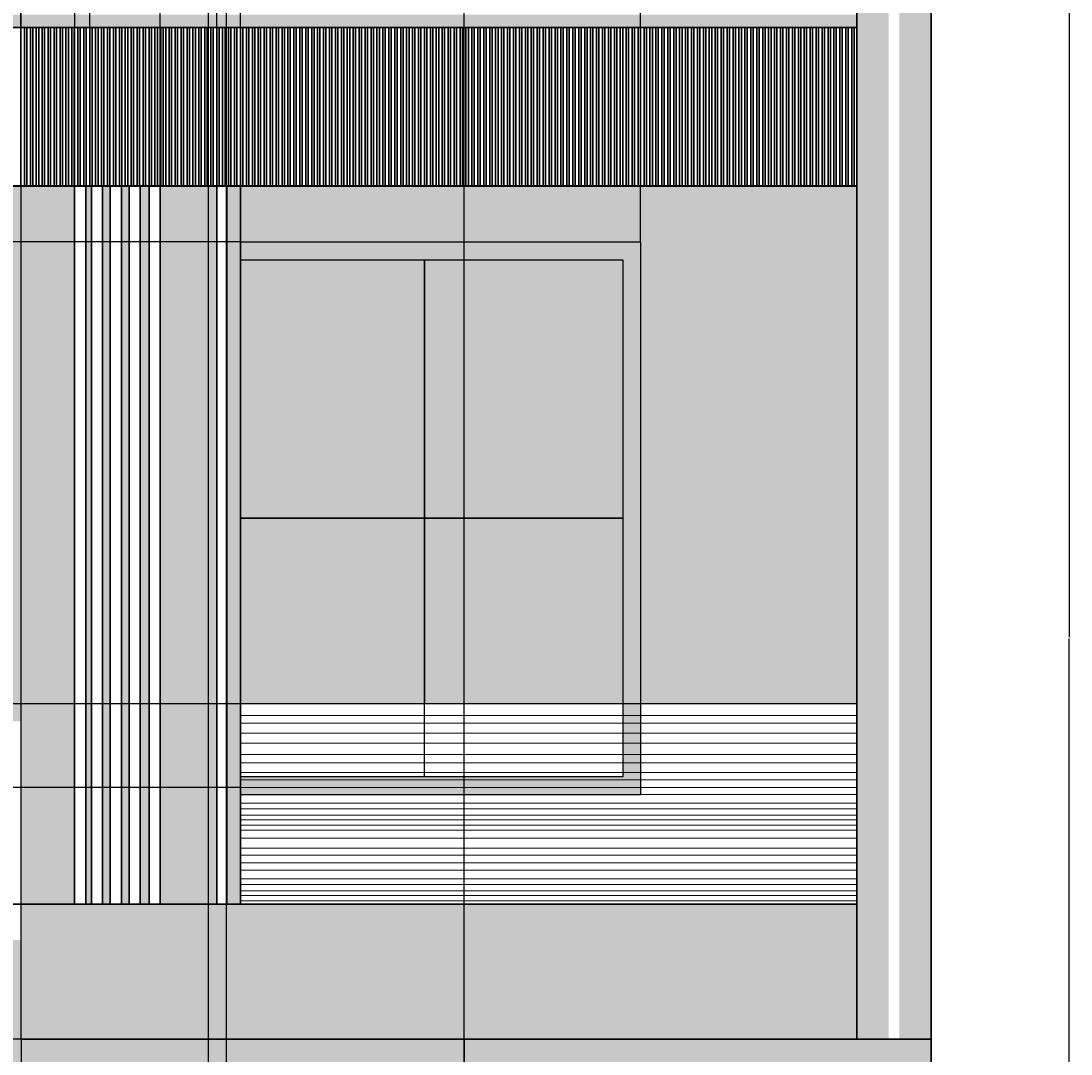
# Model space of a CAD drawing. Units: feet. Extents: x 2368 to 2738, y 1285 to 1782.
# Tile 5 of 6: x 2561 to 2738, y 1464 to 1638. Entities that reach past the tile are written whole.
import ezdxf

# ---------------------------------------------------------------- set-up
doc = ezdxf.new("R2010")
doc.units = ezdxf.units.FT
for name, color, linetype, lineweight in [('A-ANNO-DIMS', 2, 'Continuous', 18), ('A-ELEV', 7, 'Continuous', 35), ('A-ELEV-PATT', 252, 'Continuous', 13), ('A-FLOR-HRAL', 8, 'Continuous', 18), ('A-GLAZ', 4, 'Continuous', 25)]:
    doc.layers.add(name, color=color, linetype=linetype, lineweight=lineweight)
doc.styles.get("Standard").update_dxf_attribs({"font": 'arial.ttf'})
doc.dimstyles.get("Standard").update_dxf_attribs({"dimtxt": 0.18, "dimasz": 0.18, "dimexe": 0.18, "dimexo": 0.0625, "dimgap": 0.09, "dimtad": 0, "dimtih": 1, "dimtoh": 1, "dimdec": 1, "dimzin": 0, "dimdsep": 46, "dimlunit": 3, "dimtxsty": 'Standard', "dimcen": 0.09, "dimadec": 0, "dimazin": 0, "dimtfac": 1, "dimtdec": 1, "dimtofl": 0, "dimtmove": 0, "dimatfit": 3, "dimfxl": 1, "dimtolj": 1, "dimtzin": 0, "dimarcsym": 0})

# ---------------------------------------------------------------- blocks, each defined once
blk = doc.blocks.new('*D2')
at = {"layer": 'A-ANNO-DIMS', "color": 0, "lineweight": -2, "transparency": 16777216}
for p, q in [((2714.23, 1758.68), (2737.59, 1758.68)), ((2737.41, 1758.5), (2737.41, 1533.95)), ((2737.41, 1309.04), (2737.41, 1533.58)), ((2714.23, 1308.86), (2737.59, 1308.86))]:
    blk.add_line(p, q, dxfattribs=at)
at = {"layer": 'A-ANNO-DIMS', "color": 0, "transparency": 16777216}
for points in [[(2737.38, 1758.5), (2737.44, 1758.5), (2737.41, 1758.68)], [(2737.38, 1309.04), (2737.44, 1309.04), (2737.41, 1308.86)]]:
    blk.add_solid(points, dxfattribs=at)
at = {"layer": 'Defpoints', "color": 0, "transparency": 16777216}
for p in [(2714.16, 1758.68), (2737.41, 1758.68), (2714.16, 1308.86)]:
    blk.add_point(p, dxfattribs=at)
at = {"layer": 'A-ANNO-DIMS', "color": 0, "transparency": 16777216, "insert": (2737.41, 1533.77), "char_height": 0.18, "attachment_point": 5}
blk.add_mtext('\\A1;449.8', dxfattribs=at)
blk = doc.blocks.new('*D19')
at = {"layer": 'A-ANNO-DIMS', "color": 0, "lineweight": -2, "transparency": 16777216}
for p, q in [((2560.8, 1466.04), (2560.8, 1285.43)), ((2543.45, 1350.79), (2543.45, 1285.43)), ((2543.63, 1285.61), (2551.74, 1285.61)), ((2560.62, 1285.61), (2552.51, 1285.61))]:
    blk.add_line(p, q, dxfattribs=at)
at = {"layer": 'A-ANNO-DIMS', "color": 0, "transparency": 16777216}
for points in [[(2543.63, 1285.64), (2543.63, 1285.58), (2543.45, 1285.61)], [(2560.62, 1285.64), (2560.62, 1285.58), (2560.8, 1285.61)]]:
    blk.add_solid(points, dxfattribs=at)
at = {"layer": 'Defpoints', "color": 0, "transparency": 16777216}
for p in [(2560.8, 1466.1), (2543.45, 1350.86), (2560.8, 1285.61)]:
    blk.add_point(p, dxfattribs=at)
at = {"layer": 'A-ANNO-DIMS', "color": 0, "transparency": 16777216, "insert": (2552.12, 1285.61), "char_height": 0.18, "attachment_point": 5}
blk.add_mtext('\\A1;17.35', dxfattribs=at)
blk = doc.blocks.new('*D20')
at = {"layer": 'A-ANNO-DIMS', "color": 0, "lineweight": -2, "transparency": 16777216}
for p, q in [((2560.8, 1466.04), (2560.8, 1285.43)), ((2592.41, 1367.92), (2592.41, 1285.43)), ((2560.98, 1285.61), (2576.21, 1285.61)), ((2592.23, 1285.61), (2577, 1285.61))]:
    blk.add_line(p, q, dxfattribs=at)
at = {"layer": 'A-ANNO-DIMS', "color": 0, "transparency": 16777216}
for points in [[(2560.98, 1285.64), (2560.98, 1285.58), (2560.8, 1285.61)], [(2592.23, 1285.64), (2592.23, 1285.58), (2592.41, 1285.61)]]:
    blk.add_solid(points, dxfattribs=at)
at = {"layer": 'Defpoints', "color": 0, "transparency": 16777216}
for p in [(2560.8, 1466.1), (2592.41, 1367.98), (2592.41, 1285.61)]:
    blk.add_point(p, dxfattribs=at)
at = {"layer": 'A-ANNO-DIMS', "color": 0, "transparency": 16777216, "insert": (2576.6, 1285.61), "char_height": 0.18, "attachment_point": 5}
blk.add_mtext('\\A1;31.62', dxfattribs=at)
blk = doc.blocks.new('*D33')
at = {"layer": 'A-ANNO-DIMS', "color": 0, "lineweight": -2, "transparency": 16777216}
for p, q in [((2592.41, 1461.2), (2592.41, 1782.11)), ((2592.59, 1781.93), (2593.76, 1781.93)), ((2595.23, 1781.93), (2594.06, 1781.93)), ((2595.41, 1458.2), (2595.41, 1782.11))]:
    blk.add_line(p, q, dxfattribs=at)
at = {"layer": 'A-ANNO-DIMS', "color": 0, "transparency": 16777216}
for points in [[(2592.59, 1781.96), (2592.59, 1781.9), (2592.41, 1781.93)], [(2595.23, 1781.96), (2595.23, 1781.9), (2595.41, 1781.93)]]:
    blk.add_solid(points, dxfattribs=at)
at = {"layer": 'Defpoints', "color": 0, "transparency": 16777216}
for p in [(2595.41, 1781.93), (2592.41, 1461.14), (2595.41, 1458.14)]:
    blk.add_point(p, dxfattribs=at)
at = {"layer": 'A-ANNO-DIMS', "color": 0, "transparency": 16777216, "insert": (2593.91, 1781.93), "char_height": 0.18, "attachment_point": 5}
blk.add_mtext('\\A1;3', dxfattribs=at)
blk = doc.blocks.new('*D34')
at = {"layer": 'A-ANNO-DIMS', "color": 0, "lineweight": -2, "transparency": 16777216}
for p, q in [((2560.8, 1466.16), (2560.8, 1782.11)), ((2560.98, 1781.93), (2597.75, 1781.93)), ((2635.31, 1781.93), (2598.54, 1781.93)), ((2635.49, 1466.16), (2635.49, 1782.11))]:
    blk.add_line(p, q, dxfattribs=at)
at = {"layer": 'A-ANNO-DIMS', "color": 0, "transparency": 16777216}
for points in [[(2560.98, 1781.96), (2560.98, 1781.9), (2560.8, 1781.93)], [(2635.31, 1781.96), (2635.31, 1781.9), (2635.49, 1781.93)]]:
    blk.add_solid(points, dxfattribs=at)
at = {"layer": 'Defpoints', "color": 0, "transparency": 16777216}
for p in [(2635.49, 1781.93), (2560.8, 1466.1), (2635.49, 1466.1)]:
    blk.add_point(p, dxfattribs=at)
at = {"layer": 'A-ANNO-DIMS', "color": 0, "transparency": 16777216, "insert": (2598.14, 1781.93), "char_height": 0.18, "attachment_point": 5}
blk.add_mtext('\\A1;74.69', dxfattribs=at)
blk = doc.blocks.new('*D35')
at = {"layer": 'A-ANNO-DIMS', "color": 0, "lineweight": -2, "transparency": 16777216}
for p, q in [((2635.49, 1466.16), (2635.49, 1782.11)), ((2635.67, 1781.93), (2668.18, 1781.93)), ((2701.48, 1781.93), (2668.97, 1781.93)), ((2701.66, 1466.16), (2701.66, 1782.11))]:
    blk.add_line(p, q, dxfattribs=at)
at = {"layer": 'A-ANNO-DIMS', "color": 0, "transparency": 16777216}
for points in [[(2635.67, 1781.96), (2635.67, 1781.9), (2635.49, 1781.93)], [(2701.48, 1781.96), (2701.48, 1781.9), (2701.66, 1781.93)]]:
    blk.add_solid(points, dxfattribs=at)
at = {"layer": 'Defpoints', "color": 0, "transparency": 16777216}
for p in [(2701.66, 1781.93), (2635.49, 1466.1), (2701.66, 1466.1)]:
    blk.add_point(p, dxfattribs=at)
at = {"layer": 'A-ANNO-DIMS', "color": 0, "transparency": 16777216, "insert": (2668.57, 1781.93), "char_height": 0.18, "attachment_point": 5}
blk.add_mtext('\\A1;66.17', dxfattribs=at)
blk = doc.blocks.new('*D36')
at = {"layer": 'A-ANNO-DIMS', "color": 0, "lineweight": -2, "transparency": 16777216}
for p, q in [((2701.6, 1488.86), (2368.11, 1488.86)), ((2368.29, 1488.68), (2368.29, 1477.66)), ((2368.29, 1466.28), (2368.29, 1477.3)), ((2701.6, 1466.1), (2368.11, 1466.1))]:
    blk.add_line(p, q, dxfattribs=at)
at = {"layer": 'A-ANNO-DIMS', "color": 0, "transparency": 16777216}
for points in [[(2368.26, 1488.68), (2368.32, 1488.68), (2368.29, 1488.86)], [(2368.26, 1466.28), (2368.32, 1466.28), (2368.29, 1466.1)]]:
    blk.add_solid(points, dxfattribs=at)
at = {"layer": 'Defpoints', "color": 0, "transparency": 16777216}
for p in [(2368.29, 1488.86), (2701.66, 1488.86), (2701.66, 1466.1)]:
    blk.add_point(p, dxfattribs=at)
at = {"layer": 'A-ANNO-DIMS', "color": 0, "transparency": 16777216, "insert": (2368.29, 1477.48), "char_height": 0.18, "attachment_point": 5}
blk.add_mtext('\\A1;22.754', dxfattribs=at)
blk = doc.blocks.new('*D37')
at = {"layer": 'A-ANNO-DIMS', "color": 0, "lineweight": -2, "transparency": 16777216}
for p, q in [((2701.6, 1522.63), (2368.11, 1522.63)), ((2368.29, 1522.45), (2368.29, 1505.93)), ((2368.29, 1489.04), (2368.29, 1505.56)), ((2701.6, 1488.86), (2368.11, 1488.86))]:
    blk.add_line(p, q, dxfattribs=at)
at = {"layer": 'A-ANNO-DIMS', "color": 0, "transparency": 16777216}
for points in [[(2368.26, 1522.45), (2368.32, 1522.45), (2368.29, 1522.63)], [(2368.26, 1489.04), (2368.32, 1489.04), (2368.29, 1488.86)]]:
    blk.add_solid(points, dxfattribs=at)
at = {"layer": 'Defpoints', "color": 0, "transparency": 16777216}
for p in [(2368.29, 1522.63), (2701.66, 1522.63), (2701.66, 1488.86)]:
    blk.add_point(p, dxfattribs=at)
at = {"layer": 'A-ANNO-DIMS', "color": 0, "transparency": 16777216, "insert": (2368.29, 1505.74), "char_height": 0.18, "attachment_point": 5}
blk.add_mtext('\\A1;33.776', dxfattribs=at)
blk = doc.blocks.new('*D38')
at = {"layer": 'A-ANNO-DIMS', "color": 0, "lineweight": -2, "transparency": 16777216}
for p, q in [((2701.6, 1636.62), (2368.11, 1636.62)), ((2368.29, 1636.44), (2368.29, 1623.45)), ((2368.29, 1610.09), (2368.29, 1623.08)), ((2701.6, 1609.91), (2368.11, 1609.91))]:
    blk.add_line(p, q, dxfattribs=at)
at = {"layer": 'A-ANNO-DIMS', "color": 0, "transparency": 16777216}
for points in [[(2368.26, 1636.44), (2368.32, 1636.44), (2368.29, 1636.62)], [(2368.26, 1610.09), (2368.32, 1610.09), (2368.29, 1609.91)]]:
    blk.add_solid(points, dxfattribs=at)
at = {"layer": 'Defpoints', "color": 0, "transparency": 16777216}
for p in [(2368.29, 1636.62), (2701.66, 1636.62), (2701.66, 1609.91)]:
    blk.add_point(p, dxfattribs=at)
at = {"layer": 'A-ANNO-DIMS', "color": 0, "transparency": 16777216, "insert": (2368.29, 1623.26), "char_height": 0.18, "attachment_point": 5}
blk.add_mtext('\\A1;26.72', dxfattribs=at)
blk = doc.blocks.new('*D54')
at = {"layer": 'A-ANNO-DIMS', "color": 0, "lineweight": -2, "transparency": 16777216}
for p, q in [((2560.78, 1609.97), (2560.78, 1782.11)), ((2560.96, 1781.93), (2564.98, 1781.93)), ((2569.66, 1781.93), (2565.63, 1781.93)), ((2569.84, 1609.97), (2569.84, 1782.11))]:
    blk.add_line(p, q, dxfattribs=at)
at = {"layer": 'A-ANNO-DIMS', "color": 0, "transparency": 16777216}
for points in [[(2560.96, 1781.96), (2560.96, 1781.9), (2560.78, 1781.93)], [(2569.66, 1781.96), (2569.66, 1781.9), (2569.84, 1781.93)]]:
    blk.add_solid(points, dxfattribs=at)
at = {"layer": 'Defpoints', "color": 0, "transparency": 16777216}
for p in [(2569.84, 1781.93), (2560.78, 1609.91), (2569.84, 1609.91)]:
    blk.add_point(p, dxfattribs=at)
at = {"layer": 'A-ANNO-DIMS', "color": 0, "transparency": 16777216, "insert": (2565.31, 1781.93), "char_height": 0.18, "attachment_point": 5}
blk.add_mtext('\\A1;9.06', dxfattribs=at)
blk = doc.blocks.new('*D55')
at = {"layer": 'A-ANNO-DIMS', "color": 0, "lineweight": -2, "transparency": 16777216}
for p, q in [((2569.84, 1609.97), (2569.84, 1782.11)), ((2570.02, 1781.93), (2576.72, 1781.93)), ((2584.06, 1781.93), (2577.35, 1781.93)), ((2584.24, 1609.97), (2584.24, 1782.11))]:
    blk.add_line(p, q, dxfattribs=at)
at = {"layer": 'A-ANNO-DIMS', "color": 0, "transparency": 16777216}
for points in [[(2570.02, 1781.96), (2570.02, 1781.9), (2569.84, 1781.93)], [(2584.06, 1781.96), (2584.06, 1781.9), (2584.24, 1781.93)]]:
    blk.add_solid(points, dxfattribs=at)
at = {"layer": 'Defpoints', "color": 0, "transparency": 16777216}
for p in [(2584.24, 1781.93), (2569.84, 1609.91), (2584.24, 1609.91)]:
    blk.add_point(p, dxfattribs=at)
at = {"layer": 'A-ANNO-DIMS', "color": 0, "transparency": 16777216, "insert": (2577.04, 1781.93), "char_height": 0.18, "attachment_point": 5}
blk.add_mtext('\\A1;14.4', dxfattribs=at)
blk = doc.blocks.new('*D56')
at = {"layer": 'A-ANNO-DIMS', "color": 0, "lineweight": -2, "transparency": 16777216}
for p, q in [((2593.78, 1609.97), (2593.78, 1782.11)), ((2593.96, 1781.93), (2595.62, 1781.93)), ((2597.6, 1781.93), (2595.93, 1781.93)), ((2597.78, 1609.97), (2597.78, 1782.11))]:
    blk.add_line(p, q, dxfattribs=at)
at = {"layer": 'A-ANNO-DIMS', "color": 0, "transparency": 16777216}
for points in [[(2593.96, 1781.96), (2593.96, 1781.9), (2593.78, 1781.93)], [(2597.6, 1781.96), (2597.6, 1781.9), (2597.78, 1781.93)]]:
    blk.add_solid(points, dxfattribs=at)
at = {"layer": 'Defpoints', "color": 0, "transparency": 16777216}
for p in [(2597.78, 1781.93), (2593.78, 1609.91), (2597.78, 1609.91)]:
    blk.add_point(p, dxfattribs=at)
at = {"layer": 'A-ANNO-DIMS', "color": 0, "transparency": 16777216, "insert": (2595.78, 1781.93), "char_height": 0.18, "attachment_point": 5}
blk.add_mtext('\\A1;4', dxfattribs=at)
blk = doc.blocks.new('*D57')
at = {"layer": 'A-ANNO-DIMS', "color": 0, "lineweight": -2, "transparency": 16777216}
for p, q in [((2569.84, 1609.97), (2569.84, 1782.11)), ((2570.02, 1781.93), (2570.71, 1781.93)), ((2572.19, 1781.93), (2571.5, 1781.93)), ((2572.37, 1609.97), (2572.37, 1782.11))]:
    blk.add_line(p, q, dxfattribs=at)
at = {"layer": 'A-ANNO-DIMS', "color": 0, "transparency": 16777216}
for points in [[(2570.02, 1781.96), (2570.02, 1781.9), (2569.84, 1781.93)], [(2572.19, 1781.96), (2572.19, 1781.9), (2572.37, 1781.93)]]:
    blk.add_solid(points, dxfattribs=at)
at = {"layer": 'Defpoints', "color": 0, "transparency": 16777216}
for p in [(2572.37, 1781.93), (2569.84, 1609.91), (2572.37, 1609.91)]:
    blk.add_point(p, dxfattribs=at)
at = {"layer": 'A-ANNO-DIMS', "color": 0, "transparency": 16777216, "insert": (2571.11, 1781.93), "char_height": 0.18, "attachment_point": 5}
blk.add_mtext('\\A1;2.539', dxfattribs=at)
blk = doc.blocks.new('*D58')
at = {"layer": 'A-ANNO-DIMS', "color": 0, "lineweight": -2, "transparency": 16777216}
for p, q in [((2597.78, 1600.54), (2597.78, 1782.11)), ((2597.96, 1781.93), (2631.09, 1781.93)), ((2665.02, 1781.93), (2631.88, 1781.93)), ((2665.2, 1600.54), (2665.2, 1782.11))]:
    blk.add_line(p, q, dxfattribs=at)
at = {"layer": 'A-ANNO-DIMS', "color": 0, "transparency": 16777216}
for points in [[(2597.96, 1781.96), (2597.96, 1781.9), (2597.78, 1781.93)], [(2665.02, 1781.96), (2665.02, 1781.9), (2665.2, 1781.93)]]:
    blk.add_solid(points, dxfattribs=at)
at = {"layer": 'Defpoints', "color": 0, "transparency": 16777216}
for p in [(2665.2, 1781.93), (2597.78, 1600.48), (2665.2, 1600.48)]:
    blk.add_point(p, dxfattribs=at)
at = {"layer": 'A-ANNO-DIMS', "color": 0, "transparency": 16777216, "insert": (2631.49, 1781.93), "char_height": 0.18, "attachment_point": 5}
blk.add_mtext('\\A1;67.42', dxfattribs=at)
blk = doc.blocks.new('*D59')
at = {"layer": 'A-ANNO-DIMS', "color": 0, "lineweight": -2, "transparency": 16777216}
for p, q in [((2665.2, 1600.54), (2665.2, 1782.11)), ((2665.38, 1781.93), (2683.03, 1781.93)), ((2701.48, 1781.93), (2683.82, 1781.93)), ((2701.66, 1609.97), (2701.66, 1782.11))]:
    blk.add_line(p, q, dxfattribs=at)
at = {"layer": 'A-ANNO-DIMS', "color": 0, "transparency": 16777216}
for points in [[(2665.38, 1781.96), (2665.38, 1781.9), (2665.2, 1781.93)], [(2701.48, 1781.96), (2701.48, 1781.9), (2701.66, 1781.93)]]:
    blk.add_solid(points, dxfattribs=at)
at = {"layer": 'Defpoints', "color": 0, "transparency": 16777216}
for p in [(2701.66, 1781.93), (2701.66, 1609.91), (2665.2, 1600.48)]:
    blk.add_point(p, dxfattribs=at)
at = {"layer": 'A-ANNO-DIMS', "color": 0, "transparency": 16777216, "insert": (2683.43, 1781.93), "char_height": 0.18, "attachment_point": 5}
blk.add_mtext('\\A1;36.46', dxfattribs=at)
blk = doc.blocks.new('*D60')
at = {"layer": 'A-ANNO-DIMS', "color": 0, "lineweight": -2, "transparency": 16777216}
for p, q in [((2597.71, 1600.48), (2368.11, 1600.48)), ((2368.29, 1600.3), (2368.29, 1554.7)), ((2368.29, 1508.74), (2368.29, 1554.34)), ((2597.71, 1508.56), (2368.11, 1508.56))]:
    blk.add_line(p, q, dxfattribs=at)
at = {"layer": 'A-ANNO-DIMS', "color": 0, "transparency": 16777216}
for points in [[(2368.26, 1600.3), (2368.32, 1600.3), (2368.29, 1600.48)], [(2368.26, 1508.74), (2368.32, 1508.74), (2368.29, 1508.56)]]:
    blk.add_solid(points, dxfattribs=at)
at = {"layer": 'Defpoints', "color": 0, "transparency": 16777216}
for p in [(2368.29, 1600.48), (2597.78, 1600.48), (2597.78, 1508.56)]:
    blk.add_point(p, dxfattribs=at)
at = {"layer": 'A-ANNO-DIMS', "color": 0, "transparency": 16777216, "insert": (2368.29, 1554.52), "char_height": 0.18, "attachment_point": 5}
blk.add_mtext('\\A1;91.92', dxfattribs=at)

msp = doc.modelspace()

# ---------------------------------------------------------------- hatches: boundary and pattern name
at = {"layer": 'A-ELEV-PATT'}
h = msp.add_hatch(color=256, dxfattribs=at)
h.set_gradient(color1=(192, 192, 192), color2=(192, 192, 192), tint=1)
h.paths.add_polyline_path([(2714.1625, 1758.6751), (2519.621, 1758.6751), (2519.621, 1716.8552), (2714.1625, 1716.8552)])
h.paths.add_polyline_path([(2701.6591, 1693.9847), (2714.1625, 1693.9847), (2714.1625, 1710.8552), (2519.621, 1710.8552), (2519.621, 1662.8552), (2592.4132, 1662.8552), (2592.4132, 1689.493), (2665.1962, 1689.493), (2665.1962, 1662.8552), (2701.6591, 1662.8552)])
h.paths.add_polyline_path([(2701.6591, 1609.9058), (2597.776, 1609.9058), (2597.776, 1600.4784), (2665.1962, 1600.4784), (2665.1962, 1596.3371), (2665.1962, 1522.6314), (2701.6591, 1522.6314)])
h.paths.add_polyline_path([(2463.0324, 1598.097), (2536.677, 1598.097), (2536.677, 1519.7115), (2560.74, 1519.7115), (2560.5754, 1609.9058), (2542.3749, 1609.9058), (2441.2488, 1609.9058), (2441.2488, 1519.7115), (2463.0324, 1519.7115)])
h.paths.add_polyline_path([(2506.1956, 1662.8552), (2391.5414, 1662.8552), (2391.5414, 1644.4206), (2438.815, 1644.4206, -0.34592239), (2445.9507, 1638.8128), (2506.1956, 1638.8128)])
h.paths.add_polyline_path([(2410.9473, 1609.9058, -0.04175491), (2411.9608, 1614.8552), (2391.5414, 1614.8552), (2391.5414, 1488.8552), (2410.9473, 1488.8552)])
h.paths.add_polyline_path([(2426.5897, 1605.0962, 1), (2422.7862, 1605.0962), (2422.7862, 1509.5049, 1), (2426.5897, 1509.5049)])
h.paths.add_polyline_path([(2463.0324, 1460.097), (2536.677, 1460.097), (2536.677, 1350.8552), (2543.4468, 1350.8552), (2543.4468, 1482.8552), (2391.5414, 1482.8552), (2391.5414, 1350.8552), (2463.0324, 1350.8552)])
h.paths.add_polyline_path([(2436.8485, 1456.084), (2436.8485, 1379.669), (2399.9065, 1379.669), (2399.9065, 1456.084)], flags=16)
h.paths.add_polyline_path([(2434.8485, 1454.084), (2434.8485, 1381.669), (2401.9065, 1381.669), (2401.9065, 1454.084)], flags=0)
h.paths.add_polyline_path([(2714.1625, 1350.8552), (2391.5414, 1350.8552), (2391.5414, 1320.8552), (2714.1625, 1320.8552)])
h.paths.add_polyline_path([(2714.1625, 1320.8552), (2391.5414, 1320.8552), (2391.5414, 1308.8552), (2714.1625, 1308.8552)])
h = msp.add_hatch(color=256, dxfattribs=at)
h.set_gradient(color1=(128, 128, 128), color2=(128, 128, 128), tint=1)
h.paths.add_polyline_path([(2519.621, 1716.8552), (2409.5414, 1716.8552), (2409.5414, 1662.8552), (2415.5414, 1662.8552), (2415.5414, 1710.8552), (2519.621, 1710.8552)])
h.paths.add_polyline_path([(2714.1625, 1716.8552), (2519.621, 1716.8552), (2519.621, 1710.8552), (2714.1625, 1710.8552)])
h.paths.add_polyline_path([(2701.6591, 1638.8128), (2445.9507, 1638.8128, -0.0752442), (2446.1448, 1636.6235), (2542.3749, 1636.6235), (2542.776, 1636.6235), (2701.6591, 1636.6235)])
h = msp.add_hatch(color=256, dxfattribs=at)
h.set_gradient(color1=(255, 255, 255), tint=1)
h.paths.add_polyline_path([(2714.1625, 1693.9847), (2708.7975, 1693.9847), (2708.7975, 1466.101), (2714.1625, 1466.101)])
h.paths.add_polyline_path([(2707.0241, 1693.9847), (2701.6591, 1693.9847), (2701.6591, 1466.101), (2707.0241, 1466.101)])
h = msp.add_hatch(color=256, dxfattribs=at)
h.set_gradient(color1=(255, 255, 255), tint=1)
h.paths.add_polyline_path([(2595.4132, 1686.493), (2662.1962, 1686.493), (2662.1962, 1662.8552), (2665.1962, 1662.8552), (2665.1962, 1689.493), (2592.4132, 1689.493), (2592.4132, 1662.8552), (2595.4132, 1662.8552)])
h.paths.add_polyline_path([(2665.1962, 1600.4784), (2597.776, 1600.4784), (2597.776, 1597.4784), (2662.1962, 1597.4784), (2662.1962, 1510.3225), (2597.776, 1510.3225), (2597.776, 1507.3225), (2665.1962, 1507.3225)])
h.paths.add_polyline_path([(2665.1962, 1461.1396), (2592.4132, 1461.1396), (2592.4132, 1367.9838), (2665.1962, 1367.9838)])
h.paths.add_polyline_path([(2662.1962, 1458.1396), (2662.1962, 1370.9838), (2595.4132, 1370.9838), (2595.4132, 1458.1396)], flags=16)
h.paths.add_polyline_path([(2593.776, 1609.9058), (2584.2358, 1609.9058), (2584.2358, 1488.8552), (2593.776, 1488.8552)])
h.paths.add_polyline_path([(2597.776, 1609.9058), (2595.4517, 1609.9058), (2595.4517, 1488.8552), (2597.776, 1488.8552)])
h.paths.add_polyline_path([(2569.8357, 1609.9058), (2560.5754, 1609.9058), (2560.74, 1519.7115), (2560.7407, 1519.7115), (2560.7407, 1519.3328), (2560.7963, 1488.8552), (2569.8357, 1488.8552)])
h.paths.add_polyline_path([(2572.6807, 1609.9058), (2571.6967, 1609.9058), (2571.6967, 1488.8552), (2572.6807, 1488.8552)])
h.paths.add_polyline_path([(2575.8428, 1609.9058), (2574.5416, 1609.9058), (2574.5416, 1488.8552), (2575.8428, 1488.8552)])
h.paths.add_polyline_path([(2579.0308, 1609.9058), (2577.7037, 1609.9058), (2577.7037, 1488.8552), (2579.0308, 1488.8552)])
h.paths.add_polyline_path([(2582.3749, 1609.9058), (2580.8918, 1609.9058), (2580.8918, 1488.8552), (2582.3749, 1488.8552)])
h = msp.add_hatch(color=256, dxfattribs=at)
h.set_gradient(color1=(0, 255, 255), color2=(0, 255, 255), tint=1)
h.paths.add_polyline_path([(2418.2281, 1454.084), (2401.9065, 1454.084), (2401.9065, 1381.669), (2418.2281, 1381.669)])
h.paths.add_polyline_path([(2434.8485, 1454.084), (2418.5148, 1454.084), (2418.5148, 1381.669), (2434.8485, 1381.669)])
h.paths.add_polyline_path([(2662.1962, 1458.1396), (2595.4132, 1458.1396), (2595.4132, 1414.5617), (2662.1962, 1414.5617)])
h.paths.add_polyline_path([(2662.1962, 1414.5617), (2628.8047, 1414.5617), (2628.8047, 1370.9838), (2662.1962, 1370.9838)])
h.paths.add_polyline_path([(2628.8047, 1414.5617), (2595.4132, 1414.5617), (2595.4132, 1370.9838), (2628.8047, 1370.9838)])
h.paths.add_polyline_path([(2662.1962, 1597.4784), (2628.8047, 1597.4784), (2628.8047, 1553.9004), (2662.1962, 1553.9004)])
h.paths.add_polyline_path([(2628.8047, 1597.4784), (2597.776, 1597.4784), (2597.776, 1553.9004), (2628.8047, 1553.9004)])
h.paths.add_polyline_path([(2628.8047, 1553.9004), (2597.776, 1553.9004), (2597.776, 1522.6314), (2628.8047, 1522.6314)])
h.paths.add_polyline_path([(2662.1962, 1553.9004), (2628.8047, 1553.9004), (2628.8047, 1522.6314), (2662.1962, 1522.6314)])
h.paths.add_polyline_path([(2662.1962, 1686.493), (2628.8047, 1686.493), (2628.8047, 1662.8552), (2662.1962, 1662.8552)])
h.paths.add_polyline_path([(2628.8047, 1686.493), (2595.4132, 1686.493), (2595.4132, 1662.8552), (2628.8047, 1662.8552)])
h = msp.add_hatch(color=256, dxfattribs=at)
h.set_gradient(color1=(242, 242, 242), color2=(242, 242, 242), tint=1)
h.paths.add_polyline_path([(2542.3749, 1636.6235), (2440.8236, 1636.6235, 0.37790365), (2410.9473, 1609.9058), (2410.9473, 1488.8552), (2441.2488, 1488.8552), (2441.2488, 1609.9058), (2542.3749, 1609.9058)])
h.paths.add_polyline_path([(2426.5897, 1605.0962), (2426.5897, 1509.5049, -1), (2422.7862, 1509.5049), (2422.7862, 1605.0962, -1)], flags=16)
h.paths.add_polyline_path([(2441.2488, 1636.6235), (2446.1448, 1636.6235, 0.43242195), (2438.815, 1644.4206), (2391.5414, 1644.4206), (2391.5414, 1620.8552), (2391.5414, 1614.8552), (2411.9608, 1614.8552, -0.33482359)])
h.paths.add_polyline_path([(2592.4132, 1461.1396), (2635.4878, 1461.1396), (2635.4878, 1466.101), (2560.7963, 1466.101), (2560.7963, 1482.8552), (2543.4468, 1482.8552), (2543.4468, 1350.8552), (2635.4878, 1350.8552), (2635.4878, 1367.9838), (2592.4132, 1367.9838)])
h = msp.add_hatch(color=256, dxfattribs=at)
h.set_gradient(color1=(128, 128, 128), color2=(128, 128, 128), tint=1)
h.paths.add_polyline_path([(2701.6591, 1488.8552), (2560.7963, 1488.8552), (2560.7963, 1466.101), (2701.6591, 1466.101)])
h = msp.add_hatch(color=256, dxfattribs=at)
h.set_gradient(color1=(144, 103, 100), color2=(144, 103, 100), tint=1)
h.paths.add_polyline_path([(2714.1625, 1466.101), (2701.6591, 1466.101), (2635.4878, 1466.101), (2635.4878, 1461.1396), (2665.1962, 1461.1396), (2665.1962, 1367.9838), (2635.4878, 1367.9838), (2635.4878, 1350.8552), (2714.1625, 1350.8552)])

# ---------------------------------------------------------------- linework, layer by layer
at = {"layer": 'A-ELEV'}
for p, q in [((2701.6591, 1693.9847), (2701.6591, 1466.101)), ((2714.1625, 1466.101), (2714.1625, 1693.9847)), ((2446.1448, 1636.6235), (2701.6591, 1636.6235)), ((2542.3749, 1636.6235), (2701.6591, 1636.6235)), ((2441.2488, 1609.9058), (2701.6591, 1609.9058)), ((2542.3749, 1609.9058), (2701.6591, 1609.9058)), ((2597.776, 1609.9058), (2597.776, 1488.8552)), ((2391.5414, 1488.8552), (2701.6591, 1488.8552)), ((2391.5414, 1488.8552), (2701.6591, 1488.8552)), ((2560.7963, 1488.8552), (2701.6591, 1488.8552)), ((2701.6591, 1466.101), (2560.7963, 1466.101)), ((2560.7963, 1466.101), (2701.6591, 1466.101)), ((2635.4878, 1461.1396), (2635.4878, 1466.101)), ((2635.4878, 1466.101), (2635.4878, 1461.1396)), ((2701.6591, 1466.101), (2714.1625, 1466.101))]:
    msp.add_line(p, q, dxfattribs=at)
msp.add_lwpolyline([(2714.1625, 1716.8552), (2714.1625, 1308.8552)], dxfattribs=at)
for points in [[(2714.1625, 1693.9847), (2701.6591, 1693.9847), (2701.6591, 1466.101), (2714.1625, 1466.101)], [(2561.3749, 1636.6235), (2561.776, 1636.6235), (2561.776, 1609.9058), (2561.3749, 1609.9058)], [(2562.3749, 1636.6235), (2562.776, 1636.6235), (2562.776, 1609.9058), (2562.3749, 1609.9058)], [(2563.3749, 1636.6235), (2563.776, 1636.6235), (2563.776, 1609.9058), (2563.3749, 1609.9058)], [(2564.3749, 1636.6235), (2564.776, 1636.6235), (2564.776, 1609.9058), (2564.3749, 1609.9058)], [(2565.3749, 1636.6235), (2565.776, 1636.6235), (2565.776, 1609.9058), (2565.3749, 1609.9058)], [(2566.3749, 1636.6235), (2566.776, 1636.6235), (2566.776, 1609.9058), (2566.3749, 1609.9058)], [(2567.3749, 1636.6235), (2567.776, 1636.6235), (2567.776, 1609.9058), (2567.3749, 1609.9058)], [(2568.3749, 1636.6235), (2568.776, 1636.6235), (2568.776, 1609.9058), (2568.3749, 1609.9058)], [(2569.3749, 1636.6235), (2569.776, 1636.6235), (2569.776, 1609.9058), (2569.3749, 1609.9058)], [(2570.3749, 1636.6235), (2570.776, 1636.6235), (2570.776, 1609.9058), (2570.3749, 1609.9058)], [(2571.3749, 1636.6235), (2571.776, 1636.6235), (2571.776, 1609.9058), (2571.3749, 1609.9058)], [(2572.3749, 1636.6235), (2572.776, 1636.6235), (2572.776, 1609.9058), (2572.3749, 1609.9058)], [(2573.3749, 1636.6235), (2573.776, 1636.6235), (2573.776, 1609.9058), (2573.3749, 1609.9058)], [(2574.3749, 1636.6235), (2574.776, 1636.6235), (2574.776, 1609.9058), (2574.3749, 1609.9058)], [(2575.3749, 1636.6235), (2575.776, 1636.6235), (2575.776, 1609.9058), (2575.3749, 1609.9058)], [(2576.3749, 1636.6235), (2576.776, 1636.6235), (2576.776, 1609.9058), (2576.3749, 1609.9058)], [(2577.3749, 1636.6235), (2577.776, 1636.6235), (2577.776, 1609.9058), (2577.3749, 1609.9058)], [(2578.3749, 1636.6235), (2578.776, 1636.6235), (2578.776, 1609.9058), (2578.3749, 1609.9058)], [(2579.3749, 1636.6235), (2579.776, 1636.6235), (2579.776, 1609.9058), (2579.3749, 1609.9058)], [(2580.3749, 1636.6235), (2580.776, 1636.6235), (2580.776, 1609.9058), (2580.3749, 1609.9058)], [(2581.3749, 1636.6235), (2581.776, 1636.6235), (2581.776, 1609.9058), (2581.3749, 1609.9058)], [(2582.3749, 1636.6235), (2582.776, 1636.6235), (2582.776, 1609.9058), (2582.3749, 1609.9058)], [(2583.3749, 1636.6235), (2583.776, 1636.6235), (2583.776, 1609.9058), (2583.3749, 1609.9058)], [(2584.3749, 1636.6235), (2584.776, 1636.6235), (2584.776, 1609.9058), (2584.3749, 1609.9058)], [(2584.776, 1636.6235), (2585.1771, 1636.6235), (2585.1771, 1609.9058), (2584.776, 1609.9058)], [(2585.776, 1636.6235), (2586.1771, 1636.6235), (2586.1771, 1609.9058), (2585.776, 1609.9058)], [(2586.776, 1636.6235), (2587.1771, 1636.6235), (2587.1771, 1609.9058), (2586.776, 1609.9058)], [(2587.776, 1636.6235), (2588.1771, 1636.6235), (2588.1771, 1609.9058), (2587.776, 1609.9058)], [(2588.776, 1636.6235), (2589.1771, 1636.6235), (2589.1771, 1609.9058), (2588.776, 1609.9058)], [(2589.776, 1636.6235), (2590.1771, 1636.6235), (2590.1771, 1609.9058), (2589.776, 1609.9058)], [(2590.776, 1636.6235), (2591.1771, 1636.6235), (2591.1771, 1609.9058), (2590.776, 1609.9058)], [(2591.776, 1636.6235), (2592.1771, 1636.6235), (2592.1771, 1609.9058), (2591.776, 1609.9058)], [(2592.776, 1636.6235), (2593.1771, 1636.6235), (2593.1771, 1609.9058), (2592.776, 1609.9058)], [(2593.776, 1636.6235), (2594.1771, 1636.6235), (2594.1771, 1609.9058), (2593.776, 1609.9058)], [(2594.776, 1636.6235), (2595.1771, 1636.6235), (2595.1771, 1609.9058), (2594.776, 1609.9058)], [(2595.776, 1636.6235), (2596.1771, 1636.6235), (2596.1771, 1609.9058), (2595.776, 1609.9058)], [(2596.776, 1636.6235), (2597.1771, 1636.6235), (2597.1771, 1609.9058), (2596.776, 1609.9058)], [(2597.776, 1636.6235), (2598.1771, 1636.6235), (2598.1771, 1609.9058), (2597.776, 1609.9058)], [(2598.776, 1636.6235), (2599.1771, 1636.6235), (2599.1771, 1609.9058), (2598.776, 1609.9058)], [(2599.776, 1636.6235), (2600.1771, 1636.6235), (2600.1771, 1609.9058), (2599.776, 1609.9058)], [(2600.776, 1636.6235), (2601.1771, 1636.6235), (2601.1771, 1609.9058), (2600.776, 1609.9058)], [(2601.776, 1636.6235), (2602.1771, 1636.6235), (2602.1771, 1609.9058), (2601.776, 1609.9058)], [(2602.776, 1636.6235), (2603.1771, 1636.6235), (2603.1771, 1609.9058), (2602.776, 1609.9058)], [(2603.776, 1636.6235), (2604.1771, 1636.6235), (2604.1771, 1609.9058), (2603.776, 1609.9058)], [(2604.776, 1636.6235), (2605.1771, 1636.6235), (2605.1771, 1609.9058), (2604.776, 1609.9058)], [(2605.776, 1636.6235), (2606.1771, 1636.6235), (2606.1771, 1609.9058), (2605.776, 1609.9058)], [(2606.776, 1636.6235), (2607.1771, 1636.6235), (2607.1771, 1609.9058), (2606.776, 1609.9058)], [(2607.776, 1636.6235), (2608.1771, 1636.6235), (2608.1771, 1609.9058), (2607.776, 1609.9058)], [(2608.776, 1636.6235), (2609.1771, 1636.6235), (2609.1771, 1609.9058), (2608.776, 1609.9058)], [(2609.776, 1636.6235), (2610.1771, 1636.6235), (2610.1771, 1609.9058), (2609.776, 1609.9058)], [(2610.776, 1636.6235), (2611.1771, 1636.6235), (2611.1771, 1609.9058), (2610.776, 1609.9058)], [(2611.776, 1636.6235), (2612.1771, 1636.6235), (2612.1771, 1609.9058), (2611.776, 1609.9058)], [(2612.776, 1636.6235), (2613.1771, 1636.6235), (2613.1771, 1609.9058), (2612.776, 1609.9058)], [(2613.776, 1636.6235), (2614.1771, 1636.6235), (2614.1771, 1609.9058), (2613.776, 1609.9058)], [(2614.776, 1636.6235), (2615.1771, 1636.6235), (2615.1771, 1609.9058), (2614.776, 1609.9058)], [(2615.776, 1636.6235), (2616.1771, 1636.6235), (2616.1771, 1609.9058), (2615.776, 1609.9058)], [(2616.776, 1636.6235), (2617.1771, 1636.6235), (2617.1771, 1609.9058), (2616.776, 1609.9058)], [(2617.776, 1636.6235), (2618.1771, 1636.6235), (2618.1771, 1609.9058), (2617.776, 1609.9058)], [(2618.776, 1636.6235), (2619.1771, 1636.6235), (2619.1771, 1609.9058), (2618.776, 1609.9058)], [(2619.776, 1636.6235), (2620.1771, 1636.6235), (2620.1771, 1609.9058), (2619.776, 1609.9058)], [(2620.776, 1636.6235), (2621.1771, 1636.6235), (2621.1771, 1609.9058), (2620.776, 1609.9058)], [(2621.776, 1636.6235), (2622.1771, 1636.6235), (2622.1771, 1609.9058), (2621.776, 1609.9058)], [(2622.776, 1636.6235), (2623.1771, 1636.6235), (2623.1771, 1609.9058), (2622.776, 1609.9058)], [(2623.776, 1636.6235), (2624.1771, 1636.6235), (2624.1771, 1609.9058), (2623.776, 1609.9058)], [(2624.776, 1636.6235), (2625.1771, 1636.6235), (2625.1771, 1609.9058), (2624.776, 1609.9058)], [(2625.776, 1636.6235), (2626.1771, 1636.6235), (2626.1771, 1609.9058), (2625.776, 1609.9058)], [(2626.776, 1636.6235), (2627.1771, 1636.6235), (2627.1771, 1609.9058), (2626.776, 1609.9058)], [(2627.776, 1636.6235), (2628.1771, 1636.6235), (2628.1771, 1609.9058), (2627.776, 1609.9058)], [(2628.776, 1636.6235), (2629.1771, 1636.6235), (2629.1771, 1609.9058), (2628.776, 1609.9058)], [(2629.776, 1636.6235), (2630.1771, 1636.6235), (2630.1771, 1609.9058), (2629.776, 1609.9058)], [(2630.776, 1636.6235), (2631.1771, 1636.6235), (2631.1771, 1609.9058), (2630.776, 1609.9058)], [(2631.776, 1636.6235), (2632.1771, 1636.6235), (2632.1771, 1609.9058), (2631.776, 1609.9058)], [(2632.776, 1636.6235), (2633.1771, 1636.6235), (2633.1771, 1609.9058), (2632.776, 1609.9058)], [(2633.776, 1636.6235), (2634.1771, 1636.6235), (2634.1771, 1609.9058), (2633.776, 1609.9058)], [(2634.776, 1636.6235), (2635.1771, 1636.6235), (2635.1771, 1609.9058), (2634.776, 1609.9058)], [(2635.776, 1636.6235), (2636.1771, 1636.6235), (2636.1771, 1609.9058), (2635.776, 1609.9058)], [(2636.776, 1636.6235), (2637.1771, 1636.6235), (2637.1771, 1609.9058), (2636.776, 1609.9058)], [(2637.776, 1636.6235), (2638.1771, 1636.6235), (2638.1771, 1609.9058), (2637.776, 1609.9058)], [(2638.776, 1636.6235), (2639.1771, 1636.6235), (2639.1771, 1609.9058), (2638.776, 1609.9058)], [(2639.776, 1636.6235), (2640.1771, 1636.6235), (2640.1771, 1609.9058), (2639.776, 1609.9058)], [(2640.776, 1636.6235), (2641.1771, 1636.6235), (2641.1771, 1609.9058), (2640.776, 1609.9058)], [(2641.776, 1636.6235), (2642.1771, 1636.6235), (2642.1771, 1609.9058), (2641.776, 1609.9058)], [(2642.776, 1636.6235), (2643.1771, 1636.6235), (2643.1771, 1609.9058), (2642.776, 1609.9058)], [(2643.776, 1636.6235), (2644.1771, 1636.6235), (2644.1771, 1609.9058), (2643.776, 1609.9058)], [(2644.776, 1636.6235), (2645.1771, 1636.6235), (2645.1771, 1609.9058), (2644.776, 1609.9058)], [(2645.776, 1636.6235), (2646.1771, 1636.6235), (2646.1771, 1609.9058), (2645.776, 1609.9058)], [(2646.776, 1636.6235), (2647.1771, 1636.6235), (2647.1771, 1609.9058), (2646.776, 1609.9058)], [(2647.776, 1636.6235), (2648.1771, 1636.6235), (2648.1771, 1609.9058), (2647.776, 1609.9058)], [(2648.776, 1636.6235), (2649.1771, 1636.6235), (2649.1771, 1609.9058), (2648.776, 1609.9058)], [(2649.776, 1636.6235), (2650.1771, 1636.6235), (2650.1771, 1609.9058), (2649.776, 1609.9058)], [(2650.776, 1636.6235), (2651.1771, 1636.6235), (2651.1771, 1609.9058), (2650.776, 1609.9058)], [(2651.776, 1636.6235), (2652.1771, 1636.6235), (2652.1771, 1609.9058), (2651.776, 1609.9058)], [(2652.776, 1636.6235), (2653.1771, 1636.6235), (2653.1771, 1609.9058), (2652.776, 1609.9058)], [(2653.776, 1636.6235), (2654.1771, 1636.6235), (2654.1771, 1609.9058), (2653.776, 1609.9058)], [(2654.776, 1636.6235), (2655.1771, 1636.6235), (2655.1771, 1609.9058), (2654.776, 1609.9058)], [(2655.776, 1636.6235), (2656.1771, 1636.6235), (2656.1771, 1609.9058), (2655.776, 1609.9058)], [(2656.776, 1636.6235), (2657.1771, 1636.6235), (2657.1771, 1609.9058), (2656.776, 1609.9058)], [(2657.776, 1636.6235), (2658.1771, 1636.6235), (2658.1771, 1609.9058), (2657.776, 1609.9058)], [(2658.776, 1636.6235), (2659.1771, 1636.6235), (2659.1771, 1609.9058), (2658.776, 1609.9058)], [(2659.776, 1636.6235), (2660.1771, 1636.6235), (2660.1771, 1609.9058), (2659.776, 1609.9058)], [(2660.776, 1636.6235), (2661.1771, 1636.6235), (2661.1771, 1609.9058), (2660.776, 1609.9058)], [(2661.776, 1636.6235), (2662.1771, 1636.6235), (2662.1771, 1609.9058), (2661.776, 1609.9058)], [(2662.776, 1636.6235), (2663.1771, 1636.6235), (2663.1771, 1609.9058), (2662.776, 1609.9058)], [(2663.776, 1636.6235), (2664.1771, 1636.6235), (2664.1771, 1609.9058), (2663.776, 1609.9058)], [(2664.776, 1636.6235), (2665.1771, 1636.6235), (2665.1771, 1609.9058), (2664.776, 1609.9058)], [(2665.776, 1636.6235), (2666.1771, 1636.6235), (2666.1771, 1609.9058), (2665.776, 1609.9058)], [(2666.776, 1636.6235), (2667.1771, 1636.6235), (2667.1771, 1609.9058), (2666.776, 1609.9058)], [(2667.776, 1636.6235), (2668.1771, 1636.6235), (2668.1771, 1609.9058), (2667.776, 1609.9058)], [(2668.776, 1636.6235), (2669.1771, 1636.6235), (2669.1771, 1609.9058), (2668.776, 1609.9058)], [(2669.776, 1636.6235), (2670.1771, 1636.6235), (2670.1771, 1609.9058), (2669.776, 1609.9058)], [(2670.776, 1636.6235), (2671.1771, 1636.6235), (2671.1771, 1609.9058), (2670.776, 1609.9058)], [(2671.776, 1636.6235), (2672.1771, 1636.6235), (2672.1771, 1609.9058), (2671.776, 1609.9058)], [(2672.776, 1636.6235), (2673.1771, 1636.6235), (2673.1771, 1609.9058), (2672.776, 1609.9058)], [(2673.776, 1636.6235), (2674.1771, 1636.6235), (2674.1771, 1609.9058), (2673.776, 1609.9058)], [(2674.776, 1636.6235), (2675.1771, 1636.6235), (2675.1771, 1609.9058), (2674.776, 1609.9058)], [(2675.776, 1636.6235), (2676.1771, 1636.6235), (2676.1771, 1609.9058), (2675.776, 1609.9058)], [(2676.776, 1636.6235), (2677.1771, 1636.6235), (2677.1771, 1609.9058), (2676.776, 1609.9058)], [(2677.776, 1636.6235), (2678.1771, 1636.6235), (2678.1771, 1609.9058), (2677.776, 1609.9058)], [(2678.776, 1636.6235), (2679.1771, 1636.6235), (2679.1771, 1609.9058), (2678.776, 1609.9058)], [(2679.776, 1636.6235), (2680.1771, 1636.6235), (2680.1771, 1609.9058), (2679.776, 1609.9058)], [(2680.776, 1636.6235), (2681.1771, 1636.6235), (2681.1771, 1609.9058), (2680.776, 1609.9058)], [(2681.776, 1636.6235), (2682.1771, 1636.6235), (2682.1771, 1609.9058), (2681.776, 1609.9058)], [(2682.776, 1636.6235), (2683.1771, 1636.6235), (2683.1771, 1609.9058), (2682.776, 1609.9058)], [(2683.776, 1636.6235), (2684.1771, 1636.6235), (2684.1771, 1609.9058), (2683.776, 1609.9058)], [(2684.776, 1636.6235), (2685.1771, 1636.6235), (2685.1771, 1609.9058), (2684.776, 1609.9058)], [(2685.776, 1636.6235), (2686.1771, 1636.6235), (2686.1771, 1609.9058), (2685.776, 1609.9058)], [(2686.776, 1636.6235), (2687.1771, 1636.6235), (2687.1771, 1609.9058), (2686.776, 1609.9058)], [(2687.776, 1636.6235), (2688.1771, 1636.6235), (2688.1771, 1609.9058), (2687.776, 1609.9058)], [(2688.776, 1636.6235), (2689.1771, 1636.6235), (2689.1771, 1609.9058), (2688.776, 1609.9058)], [(2689.776, 1636.6235), (2690.1771, 1636.6235), (2690.1771, 1609.9058), (2689.776, 1609.9058)], [(2690.776, 1636.6235), (2691.1771, 1636.6235), (2691.1771, 1609.9058), (2690.776, 1609.9058)], [(2691.776, 1636.6235), (2692.1771, 1636.6235), (2692.1771, 1609.9058), (2691.776, 1609.9058)], [(2692.776, 1636.6235), (2693.1771, 1636.6235), (2693.1771, 1609.9058), (2692.776, 1609.9058)], [(2693.776, 1636.6235), (2694.1771, 1636.6235), (2694.1771, 1609.9058), (2693.776, 1609.9058)], [(2694.776, 1636.6235), (2695.1771, 1636.6235), (2695.1771, 1609.9058), (2694.776, 1609.9058)], [(2695.776, 1636.6235), (2696.1771, 1636.6235), (2696.1771, 1609.9058), (2695.776, 1609.9058)], [(2696.776, 1636.6235), (2697.1771, 1636.6235), (2697.1771, 1609.9058), (2696.776, 1609.9058)], [(2697.776, 1636.6235), (2698.1771, 1636.6235), (2698.1771, 1609.9058), (2697.776, 1609.9058)], [(2698.776, 1636.6235), (2699.1771, 1636.6235), (2699.1771, 1609.9058), (2698.776, 1609.9058)], [(2699.776, 1636.6235), (2700.1771, 1636.6235), (2700.1771, 1609.9058), (2699.776, 1609.9058)], [(2700.776, 1636.6235), (2701.1771, 1636.6235), (2701.1771, 1609.9058), (2700.776, 1609.9058)], [(2571.6967, 1488.8552), (2569.8357, 1488.8552), (2569.8357, 1609.9058), (2571.6967, 1609.9058)], [(2574.5416, 1488.8552), (2572.6807, 1488.8552), (2572.6807, 1609.9058), (2574.5416, 1609.9058)], [(2577.7037, 1488.8552), (2575.8428, 1488.8552), (2575.8428, 1609.9058), (2577.7037, 1609.9058)], [(2580.8918, 1488.8552), (2579.0308, 1488.8552), (2579.0308, 1609.9058), (2580.8918, 1609.9058)], [(2584.2358, 1488.8552), (2582.3749, 1488.8552), (2582.3749, 1609.9058), (2584.2358, 1609.9058)], [(2595.4517, 1488.8552), (2593.776, 1488.8552), (2593.776, 1609.9058), (2595.4517, 1609.9058)]]:
    msp.add_lwpolyline(points, close=True, dxfattribs=at)
at = {"layer": 'A-FLOR-HRAL'}
for p, q in [((2701.6591, 1522.6314), (2597.776, 1522.6314)), ((2701.6591, 1520.6424), (2597.776, 1520.6424)), ((2701.6591, 1519.351), (2597.776, 1519.351)), ((2701.6591, 1517.6908), (2597.776, 1517.6908)), ((2701.6591, 1516.0305), (2597.776, 1516.0305)), ((2701.6591, 1514.0935), (2597.776, 1514.0935)), ((2701.6591, 1512.71), (2597.776, 1512.71)), ((2701.6591, 1511.0497), (2597.776, 1511.0497)), ((2701.6591, 1509.8506), (2597.776, 1509.8506)), ((2701.6591, 1508.5593), (2597.776, 1508.5593)), ((2701.6591, 1507.3602), (2597.776, 1507.3602)), ((2701.6591, 1505.8844), (2597.776, 1505.8844)), ((2701.6591, 1504.9521), (2597.776, 1504.9521)), ((2701.6591, 1503.8552), (2597.776, 1503.8552)), ((2701.6591, 1503.0808), (2597.776, 1503.0808)), ((2701.6591, 1502.1684), (2597.776, 1502.1684)), ((2701.6591, 1501.3549), (2597.776, 1501.3549)), ((2701.6591, 1499.9713), (2597.776, 1499.9713)), ((2701.6591, 1498.3111), (2597.776, 1498.3111)), ((2701.6591, 1497.112), (2597.776, 1497.112)), ((2701.6591, 1495.8207), (2597.776, 1495.8207)), ((2701.6591, 1494.6216), (2597.776, 1494.6216)), ((2701.6591, 1493.1458), (2597.776, 1493.1458)), ((2701.6591, 1492.2135), (2597.776, 1492.2135)), ((2701.6591, 1491.1166), (2597.776, 1491.1166)), ((2701.6591, 1490.3422), (2597.776, 1490.3422)), ((2701.6591, 1489.4298), (2597.776, 1489.4298))]:
    msp.add_line(p, q, dxfattribs=at)
at = {"layer": 'A-GLAZ'}
for p, q in [((2628.8047, 1510.3225), (2628.8047, 1597.4784)), ((2597.776, 1553.9004), (2662.1962, 1553.9004))]:
    msp.add_line(p, q, dxfattribs=at)
for points in [[(2597.776, 1600.4784), (2665.1962, 1600.4784), (2665.1962, 1507.3225), (2597.776, 1507.3225)], [(2665.1962, 1600.4784), (2665.1962, 1596.3371)], [(2597.776, 1597.4784), (2662.1962, 1597.4784), (2662.1962, 1510.3225), (2597.776, 1510.3225)]]:
    msp.add_lwpolyline(points, dxfattribs=at)
for points in [[(2597.776, 1600.4784), (2665.1962, 1600.4784), (2665.1962, 1507.3225), (2597.776, 1507.3225)], [(2597.776, 1597.4784), (2662.1962, 1597.4784), (2662.1962, 1522.6314), (2597.776, 1522.6314)], [(2628.8047, 1597.4784), (2628.8047, 1597.4784), (2628.8047, 1522.6314), (2628.8047, 1522.6314)], [(2597.776, 1553.9004), (2662.1962, 1553.9004), (2662.1962, 1553.9004), (2597.776, 1553.9004)]]:
    msp.add_lwpolyline(points, close=True, dxfattribs=at)

# ---------------------------------------------------------------- dimensions: what is measured, and where the dimension line sits
at = {"layer": 'A-ANNO-DIMS'}
for base, p1, p2, override, picture, middle in [((2569.8357, 1781.9251), (2560.776, 1609.9058), (2569.8357, 1609.9058), {"dimdec": 2, "dimlfac": 1, "dimrnd": 0, "dimzin": 0, "dimdsep": 46, "dimlunit": 2}, '*D54', (2565.3059, 1781.9251)), ((2635.4878, 1781.9251), (2560.7963, 1466.101), (2635.4878, 1466.101), {"dimdec": 2, "dimlfac": 1, "dimrnd": 0, "dimzin": 0, "dimdsep": 46, "dimlunit": 2}, '*D34', (2598.1421, 1781.9251)), ((2584.2358, 1781.9251), (2569.8357, 1609.9058), (2584.2358, 1609.9058), {"dimdec": 1, "dimlfac": 1, "dimrnd": 0, "dimzin": 0, "dimdsep": 46, "dimlunit": 2}, '*D55', (2577.0358, 1781.9251)), ((2572.3749, 1781.9251), (2569.8357, 1609.9058), (2572.3749, 1609.9058), {"dimdec": 3, "dimlfac": 1, "dimrnd": 0, "dimzin": 0, "dimdsep": 46, "dimlunit": 2}, '*D57', (2571.1053, 1781.9251)), ((2595.4132, 1781.9251), (2592.4132, 1461.1396), (2595.4132, 1458.1396), {"dimdec": 0, "dimlfac": 1, "dimrnd": 0, "dimzin": 0, "dimdsep": 46, "dimlunit": 2}, '*D33', (2593.9132, 1781.9251)), ((2597.776, 1781.9251), (2593.776, 1609.9058), (2597.776, 1609.9058), {"dimdec": 0, "dimlfac": 1, "dimrnd": 0, "dimzin": 0, "dimdsep": 46, "dimlunit": 2}, '*D56', (2595.776, 1781.9251)), ((2665.1962, 1781.9251), (2597.776, 1600.4784), (2665.1962, 1600.4784), {"dimdec": 2, "dimlfac": 1, "dimrnd": 0, "dimzin": 0, "dimdsep": 46, "dimlunit": 2}, '*D58', (2631.4861, 1781.9251)), ((2701.6591, 1781.9251), (2635.4878, 1466.101), (2701.6591, 1466.101), {"dimdec": 2, "dimlfac": 1, "dimrnd": 0, "dimzin": 0, "dimdsep": 46, "dimlunit": 2}, '*D35', (2668.5735, 1781.9251)), ((2701.6591, 1781.9251), (2665.1962, 1600.4784), (2701.6591, 1609.9058), {"dimdec": 2, "dimlfac": 1, "dimrnd": 0, "dimzin": 0, "dimdsep": 46, "dimlunit": 2}, '*D59', (2683.4277, 1781.9251)), ((2560.7963, 1285.6052), (2543.4468, 1350.8552), (2560.7963, 1466.101), {"dimdec": 2, "dimlfac": 1, "dimrnd": 0, "dimzin": 0, "dimdsep": 46, "dimlunit": 2}, '*D19', (2552.1216, 1285.6052)), ((2592.4132, 1285.6052), (2560.7963, 1466.101), (2592.4132, 1367.9838), {"dimdec": 2, "dimlfac": 1, "dimrnd": 0, "dimzin": 0, "dimdsep": 46, "dimlunit": 2}, '*D20', (2576.6047, 1285.6052))]:
    dim = msp.add_linear_dim(base=base, p1=p1, p2=p2, dimstyle='Standard', override=override, dxfattribs=at)
    dim.commit()
    dim.dimension.update_dxf_attribs({"geometry": picture, "text_midpoint": middle})
for base, p1, p2, override, picture, middle in [((2737.4125, 1758.6751), (2714.1625, 1308.8552), (2714.1625, 1758.6751), {"dimdec": 1, "dimlfac": 1, "dimrnd": 0, "dimzin": 0, "dimdsep": 46, "dimlunit": 2}, '*D2', (2737.4125, 1533.7652)), ((2368.2914, 1636.6235), (2701.6591, 1609.9058), (2701.6591, 1636.6235), {"dimdec": 2, "dimlfac": 1, "dimrnd": 0, "dimzin": 0, "dimdsep": 46, "dimlunit": 2}, '*D38', (2368.2914, 1623.2646)), ((2368.2914, 1600.4784), (2597.776, 1508.5593), (2597.776, 1600.4784), {"dimdec": 2, "dimlfac": 1, "dimrnd": 0, "dimzin": 0, "dimdsep": 46, "dimlunit": 2}, '*D60', (2368.2914, 1554.5188)), ((2368.2914, 1522.6314), (2701.6591, 1488.8552), (2701.6591, 1522.6314), {"dimdec": 3, "dimlfac": 1, "dimrnd": 0, "dimzin": 0, "dimdsep": 46, "dimlunit": 2}, '*D37', (2368.2914, 1505.7433)), ((2368.2914, 1488.8552), (2701.6591, 1466.101), (2701.6591, 1488.8552), {"dimdec": 3, "dimlfac": 1, "dimrnd": 0, "dimzin": 0, "dimdsep": 46, "dimlunit": 2}, '*D36', (2368.2914, 1477.4781))]:
    dim = msp.add_linear_dim(base=base, p1=p1, p2=p2, angle=90, dimstyle='Standard', override=override, dxfattribs=at)
    dim.commit()
    dim.dimension.update_dxf_attribs({"geometry": picture, "text_midpoint": middle})

doc.saveas('drawing.dxf')
